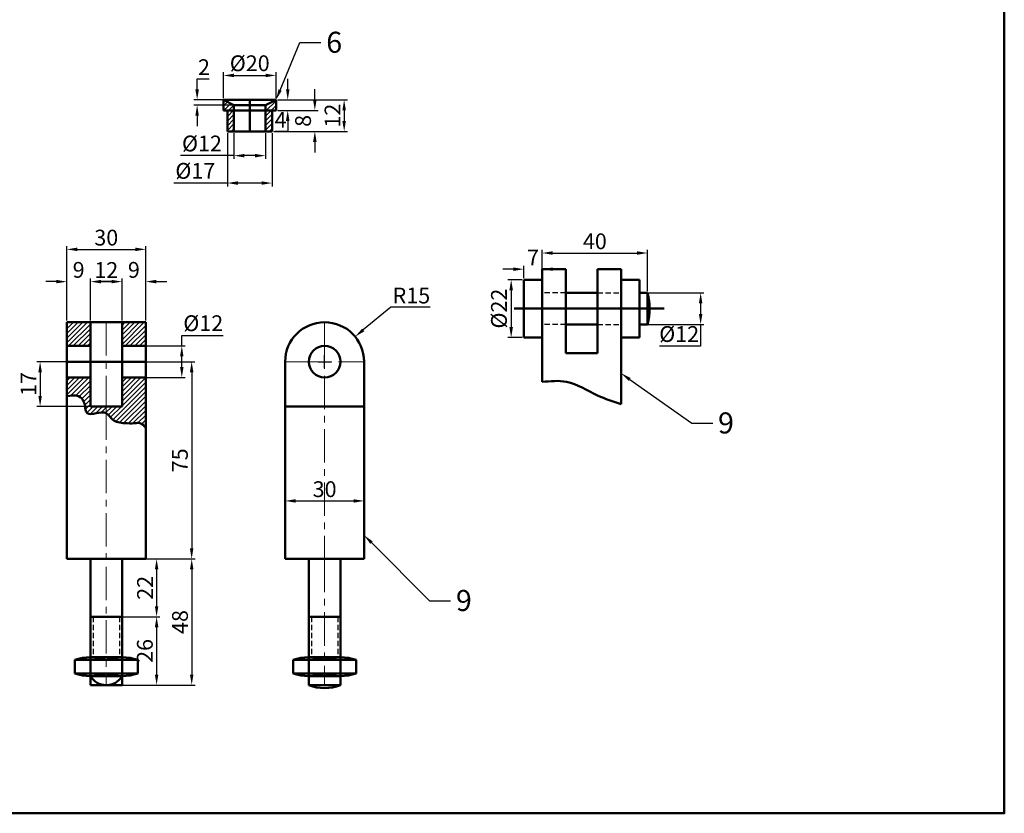
# Model space of a CAD drawing. Units: millimetres. Extents: x -266 to 493, y 251 to 855.
# Tile 2 of 3: x 118 to 493, y 251 to 553. Entities that reach past the tile are written whole.
import ezdxf
from ezdxf import colors
from ezdxf.entities.mleader import LeaderData, LeaderLine
from ezdxf.math import Vec2, Vec3

# ---------------------------------------------------------------- set-up
doc = ezdxf.new("R2010")
doc.units = ezdxf.units.MM
doc.header["$LTSCALE"] = 0.4
doc.linetypes.add('CENTER', pattern=[50.8, 31.75, -6.35, 6.35, -6.35])
doc.linetypes.add('DASHED', pattern=[19.05, 12.7, -6.35])
for name, color, linetype, lineweight in [('M-CNTR', 1, 'CENTER', 18), ('M-DIMS', 2, 'Continuous', 25), ('M-HATC', 8, 'Continuous', 18), ('M-HIDN', 3, 'DASHED', 25), ('M-OUTL', 7, 'Continuous', 50), ('M-TEXT', 7, 'Continuous', 25)]:
    doc.layers.add(name, color=color, linetype=linetype, lineweight=lineweight)
doc.styles.get("Standard").update_dxf_attribs({"font": 'arial.ttf'})
doc.dimstyles.new('ISO-25', dxfattribs={"dimtxt": 6, "dimasz": 4, "dimexe": 1.25, "dimexo": 0.625, "dimtad": 1, "dimtoh": 1, "dimtxsty": 'Standard', "dimcen": 2.5, "dimadec": 0, "dimazin": 0, "dimtfac": 1, "dimtofl": 0, "dimtmove": 0, "dimatfit": 3, "dimfxl": 1, "dimarcsym": 0})

# ---------------------------------------------------------------- blocks, each defined once
blk = doc.blocks.new('*D34')
at = {"layer": 'Defpoints', "color": 0, "transparency": 16777216}
for p in [(199.69, 510.13), (211.69, 510.13), (211.69, 500.9)]:
    blk.add_point(p, dxfattribs=at)
at = {"layer": 'M-DIMS', "color": 0, "lineweight": -2, "transparency": 16777216}
for p, q in [((199.69, 509.51), (199.69, 499.65)), ((211.69, 509.51), (211.69, 499.65)), ((199.69, 500.9), (179.38, 500.9)), ((207.69, 500.9), (203.69, 500.9))]:
    blk.add_line(p, q, dxfattribs=at)
at = {"layer": 'M-DIMS', "color": 0, "transparency": 16777216}
for points in [[(203.69, 501.57), (203.69, 500.23), (199.69, 500.9)], [(207.69, 501.57), (207.69, 500.23), (211.69, 500.9)]]:
    blk.add_solid(points, dxfattribs=at)
at = {"layer": 'M-DIMS', "color": 0, "transparency": 16777216, "insert": (187.53, 504.75), "char_height": 6, "attachment_point": 5}
blk.add_mtext('%%C12', dxfattribs=at)
blk = doc.blocks.new('*D35')
at = {"layer": 'Defpoints', "color": 0, "transparency": 16777216}
for p in [(197.19, 510.13), (214.19, 510.13), (214.19, 490.48)]:
    blk.add_point(p, dxfattribs=at)
at = {"layer": 'M-DIMS', "color": 0, "lineweight": -2, "transparency": 16777216}
for p, q in [((197.19, 509.51), (197.19, 489.23)), ((214.19, 509.51), (214.19, 489.23)), ((197.19, 490.48), (176.81, 490.48)), ((210.19, 490.48), (201.19, 490.48))]:
    blk.add_line(p, q, dxfattribs=at)
at = {"layer": 'M-DIMS', "color": 0, "transparency": 16777216}
for points in [[(201.19, 491.15), (201.19, 489.82), (197.19, 490.48)], [(210.19, 491.15), (210.19, 489.82), (214.19, 490.48)]]:
    blk.add_solid(points, dxfattribs=at)
at = {"layer": 'M-DIMS', "color": 0, "transparency": 16777216, "insert": (185, 494.34), "char_height": 6, "attachment_point": 5}
blk.add_mtext('%%C17', dxfattribs=at)
blk = doc.blocks.new('*D36')
at = {"layer": 'Defpoints', "color": 0, "transparency": 16777216}
for p in [(215.69, 522.13), (215.69, 518.13), (220.13, 518.13)]:
    blk.add_point(p, dxfattribs=at)
at = {"layer": 'M-DIMS', "color": 0, "lineweight": -2, "transparency": 16777216}
for p, q in [((220.13, 526.13), (220.13, 530.13)), ((216.31, 522.13), (221.38, 522.13)), ((216.31, 518.13), (221.38, 518.13)), ((220.13, 514.13), (220.13, 510.13)), ((220.13, 510.13), (215.36, 510.13))]:
    blk.add_line(p, q, dxfattribs=at)
at = {"layer": 'M-DIMS', "color": 0, "transparency": 16777216}
for points in [[(219.47, 526.13), (220.8, 526.13), (220.13, 522.13)], [(219.47, 514.13), (220.8, 514.13), (220.13, 518.13)]]:
    blk.add_solid(points, dxfattribs=at)
at = {"layer": 'M-DIMS', "color": 0, "transparency": 16777216, "insert": (217.43, 513.76), "char_height": 6, "attachment_point": 5}
blk.add_mtext('4', dxfattribs=at)
blk = doc.blocks.new('*D37')
at = {"layer": 'Defpoints', "color": 0, "transparency": 16777216}
for p in [(215.69, 522.13), (214.19, 510.13), (241.58, 510.13)]:
    blk.add_point(p, dxfattribs=at)
at = {"layer": 'M-DIMS', "color": 0, "lineweight": -2, "transparency": 16777216}
for p, q in [((216.31, 522.13), (242.83, 522.13)), ((241.58, 518.13), (241.58, 514.13)), ((214.81, 510.13), (242.83, 510.13))]:
    blk.add_line(p, q, dxfattribs=at)
at = {"layer": 'M-DIMS', "color": 0, "transparency": 16777216}
for points in [[(240.91, 518.13), (242.25, 518.13), (241.58, 522.13)], [(240.91, 514.13), (242.25, 514.13), (241.58, 510.13)]]:
    blk.add_solid(points, dxfattribs=at)
at = {"layer": 'M-DIMS', "color": 0, "transparency": 16777216, "insert": (237.94, 516.13), "char_height": 6, "attachment_point": 5, "rotation": 90}
blk.add_mtext('12', dxfattribs=at)
blk = doc.blocks.new('*D38')
at = {"layer": 'Defpoints', "color": 0, "transparency": 16777216}
for p in [(215.69, 518.13), (214.19, 510.13), (230.43, 510.13)]:
    blk.add_point(p, dxfattribs=at)
at = {"layer": 'M-DIMS', "color": 0, "lineweight": -2, "transparency": 16777216}
for p, q in [((230.43, 522.13), (230.43, 526.13)), ((216.31, 518.13), (231.68, 518.13)), ((214.81, 510.13), (231.68, 510.13)), ((230.43, 506.13), (230.43, 502.13))]:
    blk.add_line(p, q, dxfattribs=at)
at = {"layer": 'M-DIMS', "color": 0, "transparency": 16777216}
for points in [[(229.76, 522.13), (231.1, 522.13), (230.43, 518.13)], [(229.76, 506.13), (231.1, 506.13), (230.43, 510.13)]]:
    blk.add_solid(points, dxfattribs=at)
at = {"layer": 'M-DIMS', "color": 0, "transparency": 16777216, "insert": (226.74, 514.13), "char_height": 6, "attachment_point": 5, "rotation": 90}
blk.add_mtext('8', dxfattribs=at)
blk = doc.blocks.new('*D39')
at = {"layer": 'Defpoints', "color": 0, "transparency": 16777216}
for p in [(185.69, 522.14), (205.69, 522.14), (205.69, 520.14)]:
    blk.add_point(p, dxfattribs=at)
at = {"layer": 'M-DIMS', "color": 0, "lineweight": -2, "transparency": 16777216}
for p, q in [((185.69, 526.14), (185.69, 530.14)), ((185.69, 530.14), (190.29, 530.14)), ((205.06, 522.14), (184.44, 522.14)), ((205.06, 520.14), (184.44, 520.14)), ((185.69, 516.14), (185.69, 512.14))]:
    blk.add_line(p, q, dxfattribs=at)
at = {"layer": 'M-DIMS', "color": 0, "transparency": 16777216}
for points in [[(185.02, 526.14), (186.36, 526.14), (185.69, 522.14)], [(185.02, 516.14), (186.36, 516.14), (185.69, 520.14)]]:
    blk.add_solid(points, dxfattribs=at)
at = {"layer": 'M-DIMS', "color": 0, "transparency": 16777216, "insert": (188.3, 533.78), "char_height": 6, "attachment_point": 5}
blk.add_mtext('2', dxfattribs=at)
blk = doc.blocks.new('*D40')
at = {"layer": 'Defpoints', "color": 0, "transparency": 16777216}
for p in [(215.69, 531.4), (195.69, 522.13), (215.69, 522.13)]:
    blk.add_point(p, dxfattribs=at)
at = {"layer": 'M-DIMS', "color": 0, "lineweight": -2, "transparency": 16777216}
for p, q in [((195.69, 522.76), (195.69, 532.65)), ((215.69, 522.76), (215.69, 532.65)), ((199.69, 531.4), (211.69, 531.4))]:
    blk.add_line(p, q, dxfattribs=at)
at = {"layer": 'M-DIMS', "color": 0, "transparency": 16777216}
for points in [[(199.69, 532.07), (199.69, 530.74), (195.69, 531.4)], [(211.69, 532.07), (211.69, 530.74), (215.69, 531.4)]]:
    blk.add_solid(points, dxfattribs=at)
at = {"layer": 'M-DIMS', "color": 0, "transparency": 16777216, "insert": (205.69, 535.26), "char_height": 6, "attachment_point": 5}
blk.add_mtext('%%C20', dxfattribs=at)
blk = doc.blocks.new('*D41')
at = {"layer": 'Defpoints', "color": 0, "transparency": 16777216}
for p in [(162.53, 422.54), (162.53, 347.54), (183.62, 347.54)]:
    blk.add_point(p, dxfattribs=at)
at = {"layer": 'M-DIMS', "color": 0, "lineweight": -2, "transparency": 16777216}
for p, q in [((163.16, 422.54), (184.87, 422.54)), ((183.62, 418.54), (183.62, 351.54)), ((163.16, 347.54), (184.87, 347.54))]:
    blk.add_line(p, q, dxfattribs=at)
at = {"layer": 'M-DIMS', "color": 0, "transparency": 16777216}
for points in [[(182.95, 418.54), (184.28, 418.54), (183.62, 422.54)], [(182.95, 351.54), (184.28, 351.54), (183.62, 347.54)]]:
    blk.add_solid(points, dxfattribs=at)
at = {"layer": 'M-DIMS', "color": 0, "transparency": 16777216, "insert": (179.94, 385.04), "char_height": 6, "attachment_point": 5, "rotation": 90}
blk.add_mtext('75', dxfattribs=at)
blk = doc.blocks.new('*D42')
at = {"layer": 'Defpoints', "color": 0, "transparency": 16777216}
for p in [(151.16, 422.54), (126.01, 405.54), (151.16, 405.54)]:
    blk.add_point(p, dxfattribs=at)
at = {"layer": 'M-DIMS', "color": 0, "lineweight": -2, "transparency": 16777216}
for p, q in [((150.54, 422.54), (124.76, 422.54)), ((126.01, 418.54), (126.01, 409.54)), ((150.54, 405.54), (124.76, 405.54))]:
    blk.add_line(p, q, dxfattribs=at)
at = {"layer": 'M-DIMS', "color": 0, "transparency": 16777216}
for points in [[(125.35, 418.54), (126.68, 418.54), (126.01, 422.54)], [(125.35, 409.54), (126.68, 409.54), (126.01, 405.54)]]:
    blk.add_solid(points, dxfattribs=at)
at = {"layer": 'M-DIMS', "color": 0, "transparency": 16777216, "insert": (122.38, 414.04), "char_height": 6, "attachment_point": 5, "rotation": 90}
blk.add_mtext('17', dxfattribs=at)
blk = doc.blocks.new('*D43')
at = {"layer": 'Defpoints', "color": 0, "transparency": 16777216}
for p in [(161.66, 428.54), (179.87, 428.54), (161.66, 416.54)]:
    blk.add_point(p, dxfattribs=at)
at = {"layer": 'M-DIMS', "color": 0, "lineweight": -2, "transparency": 16777216}
for p, q in [((179.87, 428.54), (179.87, 432.54)), ((179.87, 432.54), (195.55, 432.54)), ((162.29, 428.54), (181.12, 428.54)), ((179.87, 420.54), (179.87, 424.54)), ((162.29, 416.54), (181.12, 416.54))]:
    blk.add_line(p, q, dxfattribs=at)
at = {"layer": 'M-DIMS', "color": 0, "transparency": 16777216}
for points in [[(179.2, 424.54), (180.53, 424.54), (179.87, 428.54)], [(179.2, 420.54), (180.53, 420.54), (179.87, 416.54)]]:
    blk.add_solid(points, dxfattribs=at)
at = {"layer": 'M-DIMS', "color": 0, "transparency": 16777216, "insert": (188.02, 436.4), "char_height": 6, "attachment_point": 5}
blk.add_mtext('%%C12', dxfattribs=at)
blk = doc.blocks.new('*D44')
at = {"layer": 'Defpoints', "color": 0, "transparency": 16777216}
for p in [(157.16, 347.54), (157.16, 325.54), (170.29, 325.54)]:
    blk.add_point(p, dxfattribs=at)
at = {"layer": 'M-DIMS', "color": 0, "lineweight": -2, "transparency": 16777216}
for p, q in [((157.79, 347.54), (171.54, 347.54)), ((170.29, 343.54), (170.29, 329.54)), ((157.79, 325.54), (171.54, 325.54))]:
    blk.add_line(p, q, dxfattribs=at)
at = {"layer": 'M-DIMS', "color": 0, "transparency": 16777216}
for points in [[(169.63, 343.54), (170.96, 343.54), (170.29, 347.54)], [(169.63, 329.54), (170.96, 329.54), (170.29, 325.54)]]:
    blk.add_solid(points, dxfattribs=at)
at = {"layer": 'M-DIMS', "color": 0, "transparency": 16777216, "insert": (166.66, 336.54), "char_height": 6, "attachment_point": 5, "rotation": 90}
blk.add_mtext('22', dxfattribs=at)
blk = doc.blocks.new('*D45')
at = {"layer": 'Defpoints', "color": 0, "transparency": 16777216}
for p in [(151.16, 325.54), (151.16, 299.54), (170.29, 299.54)]:
    blk.add_point(p, dxfattribs=at)
at = {"layer": 'M-DIMS', "color": 0, "lineweight": -2, "transparency": 16777216}
for p, q in [((151.79, 325.54), (171.54, 325.54)), ((170.29, 321.54), (170.29, 303.54)), ((151.79, 299.54), (171.54, 299.54))]:
    blk.add_line(p, q, dxfattribs=at)
at = {"layer": 'M-DIMS', "color": 0, "transparency": 16777216}
for points in [[(169.63, 321.54), (170.96, 321.54), (170.29, 325.54)], [(169.63, 303.54), (170.96, 303.54), (170.29, 299.54)]]:
    blk.add_solid(points, dxfattribs=at)
at = {"layer": 'M-DIMS', "color": 0, "transparency": 16777216, "insert": (166.6, 312.54), "char_height": 6, "attachment_point": 5, "rotation": 90}
blk.add_mtext('26', dxfattribs=at)
blk = doc.blocks.new('*D46')
at = {"layer": 'Defpoints', "color": 0, "transparency": 16777216}
for p in [(166.16, 347.54), (157.16, 299.54), (183.64, 299.54)]:
    blk.add_point(p, dxfattribs=at)
at = {"layer": 'M-DIMS', "color": 0, "lineweight": -2, "transparency": 16777216}
for p, q in [((166.79, 347.54), (184.89, 347.54)), ((183.64, 343.54), (183.64, 303.54)), ((157.79, 299.54), (184.89, 299.54))]:
    blk.add_line(p, q, dxfattribs=at)
at = {"layer": 'M-DIMS', "color": 0, "transparency": 16777216}
for points in [[(182.97, 343.54), (184.3, 343.54), (183.64, 347.54)], [(182.97, 303.54), (184.3, 303.54), (183.64, 299.54)]]:
    blk.add_solid(points, dxfattribs=at)
at = {"layer": 'M-DIMS', "color": 0, "transparency": 16777216, "insert": (179.95, 323.54), "char_height": 6, "attachment_point": 5, "rotation": 90}
blk.add_mtext('48', dxfattribs=at)
blk = doc.blocks.new('*D47')
at = {"layer": 'Defpoints', "color": 0, "transparency": 16777216}
for p in [(166.16, 465.26), (136.16, 437.54), (166.16, 437.54)]:
    blk.add_point(p, dxfattribs=at)
at = {"layer": 'M-DIMS', "color": 0, "lineweight": -2, "transparency": 16777216}
for p, q in [((136.16, 438.17), (136.16, 466.51)), ((140.16, 465.26), (162.16, 465.26)), ((166.16, 438.17), (166.16, 466.51))]:
    blk.add_line(p, q, dxfattribs=at)
at = {"layer": 'M-DIMS', "color": 0, "transparency": 16777216}
for points in [[(140.16, 465.93), (140.16, 464.6), (136.16, 465.26)], [(162.16, 465.93), (162.16, 464.6), (166.16, 465.26)]]:
    blk.add_solid(points, dxfattribs=at)
at = {"layer": 'M-DIMS', "color": 0, "transparency": 16777216, "insert": (151.16, 468.95), "char_height": 6, "attachment_point": 5}
blk.add_mtext('30', dxfattribs=at)
blk = doc.blocks.new('*D48')
at = {"layer": 'Defpoints', "color": 0, "transparency": 16777216}
for p in [(157.16, 452.99), (145.16, 437.54), (157.16, 437.54)]:
    blk.add_point(p, dxfattribs=at)
at = {"layer": 'M-DIMS', "color": 0, "lineweight": -2, "transparency": 16777216}
for p, q in [((145.16, 438.17), (145.16, 454.24)), ((149.16, 452.99), (153.16, 452.99)), ((157.16, 438.17), (157.16, 454.24))]:
    blk.add_line(p, q, dxfattribs=at)
at = {"layer": 'M-DIMS', "color": 0, "transparency": 16777216}
for points in [[(149.16, 453.66), (149.16, 452.33), (145.16, 452.99)], [(153.16, 453.66), (153.16, 452.33), (157.16, 452.99)]]:
    blk.add_solid(points, dxfattribs=at)
at = {"layer": 'M-DIMS', "color": 0, "transparency": 16777216, "insert": (151.16, 456.63), "char_height": 6, "attachment_point": 5}
blk.add_mtext('12', dxfattribs=at)
blk = doc.blocks.new('*D49')
at = {"layer": 'Defpoints', "color": 0, "transparency": 16777216}
for p in [(145.16, 452.99), (136.16, 437.54), (145.16, 437.54)]:
    blk.add_point(p, dxfattribs=at)
at = {"layer": 'M-DIMS', "color": 0, "lineweight": -2, "transparency": 16777216}
for p, q in [((132.16, 452.99), (128.16, 452.99)), ((136.16, 438.17), (136.16, 454.24)), ((145.16, 438.17), (145.16, 454.24)), ((149.16, 452.99), (153.16, 452.99))]:
    blk.add_line(p, q, dxfattribs=at)
at = {"layer": 'M-DIMS', "color": 0, "transparency": 16777216}
for points in [[(132.16, 453.66), (132.16, 452.33), (136.16, 452.99)], [(149.16, 453.66), (149.16, 452.33), (145.16, 452.99)]]:
    blk.add_solid(points, dxfattribs=at)
at = {"layer": 'M-DIMS', "color": 0, "transparency": 16777216, "insert": (140.66, 456.68), "char_height": 6, "attachment_point": 5}
blk.add_mtext('9', dxfattribs=at)
blk = doc.blocks.new('*D50')
at = {"layer": 'Defpoints', "color": 0, "transparency": 16777216}
for p in [(166.16, 452.99), (157.16, 437.54), (166.16, 437.54)]:
    blk.add_point(p, dxfattribs=at)
at = {"layer": 'M-DIMS', "color": 0, "lineweight": -2, "transparency": 16777216}
for p, q in [((153.16, 452.99), (149.16, 452.99)), ((157.16, 438.17), (157.16, 454.24)), ((166.16, 438.17), (166.16, 454.24)), ((170.16, 452.99), (174.16, 452.99))]:
    blk.add_line(p, q, dxfattribs=at)
at = {"layer": 'M-DIMS', "color": 0, "transparency": 16777216}
for points in [[(153.16, 453.66), (153.16, 452.33), (157.16, 452.99)], [(170.16, 453.66), (170.16, 452.33), (166.16, 452.99)]]:
    blk.add_solid(points, dxfattribs=at)
at = {"layer": 'M-DIMS', "color": 0, "transparency": 16777216, "insert": (161.66, 456.68), "char_height": 6, "attachment_point": 5}
blk.add_mtext('9', dxfattribs=at)
blk = doc.blocks.new('*D51')
at = {"layer": 'Defpoints', "color": 0, "transparency": 16777216}
for p in [(219.15, 379.25), (249.15, 379.25), (249.15, 369.59)]:
    blk.add_point(p, dxfattribs=at)
at = {"layer": 'M-DIMS', "color": 0, "lineweight": -2, "transparency": 16777216}
for p, q in [((219.15, 378.63), (219.15, 368.34)), ((249.15, 378.63), (249.15, 368.34)), ((223.15, 369.59), (245.15, 369.59))]:
    blk.add_line(p, q, dxfattribs=at)
at = {"layer": 'M-DIMS', "color": 0, "transparency": 16777216}
for points in [[(223.15, 370.25), (223.15, 368.92), (219.15, 369.59)], [(245.15, 370.25), (245.15, 368.92), (249.15, 369.59)]]:
    blk.add_solid(points, dxfattribs=at)
at = {"layer": 'M-DIMS', "color": 0, "transparency": 16777216, "insert": (234.15, 373.28), "char_height": 6, "attachment_point": 5}
blk.add_mtext('30', dxfattribs=at)
blk = doc.blocks.new('*D52')
at = {"layer": 'Defpoints', "color": 0, "transparency": 16777216}
for p in [(245.74, 432.07), (234.15, 422.54)]:
    blk.add_point(p, dxfattribs=at)
at = {"layer": 'M-DIMS', "color": 0, "lineweight": -2, "transparency": 16777216}
for p, q in [((259.32, 443.23), (248.83, 434.61)), ((274.33, 443.23), (259.32, 443.23)), ((234.15, 420.04), (234.15, 425.04)), ((231.65, 422.54), (236.65, 422.54))]:
    blk.add_line(p, q, dxfattribs=at)
at = {"layer": 'M-DIMS', "color": 0, "transparency": 16777216}
blk.add_solid([(248.41, 435.12), (249.25, 434.09), (245.74, 432.07)], dxfattribs=at)
at = {"layer": 'M-DIMS', "color": 0, "transparency": 16777216, "insert": (267.14, 446.92), "char_height": 6, "attachment_point": 5}
blk.add_mtext('R15', dxfattribs=at)
blk = doc.blocks.new('*D69')
at = {"layer": 'Defpoints', "color": 0, "ltscale": 0.4, "transparency": 16777216}
for p in [(356.87, 463.87), (316.87, 457.73), (356.87, 448.73)]:
    blk.add_point(p, dxfattribs=at)
at = {"layer": 'M-DIMS', "color": 0, "lineweight": -2, "ltscale": 0.4, "transparency": 16777216}
for p, q in [((316.87, 458.35), (316.87, 465.12)), ((356.87, 449.35), (356.87, 465.12)), ((320.87, 463.87), (352.87, 463.87))]:
    blk.add_line(p, q, dxfattribs=at)
at = {"layer": 'M-DIMS', "color": 0, "ltscale": 0.4, "transparency": 16777216}
for points in [[(320.87, 464.53), (320.87, 463.2), (316.87, 463.87)], [(352.87, 464.53), (352.87, 463.2), (356.87, 463.87)]]:
    blk.add_solid(points, dxfattribs=at)
at = {"layer": 'M-DIMS', "color": 0, "ltscale": 0.4, "transparency": 16777216, "insert": (336.87, 467.56), "char_height": 6, "attachment_point": 5}
blk.add_mtext('40', dxfattribs=at)
blk = doc.blocks.new('*D70')
at = {"layer": 'Defpoints', "color": 0, "ltscale": 0.4, "transparency": 16777216}
for p in [(316.87, 457.73), (309.87, 453.73), (316.87, 453.73)]:
    blk.add_point(p, dxfattribs=at)
at = {"layer": 'M-DIMS', "color": 0, "lineweight": -2, "ltscale": 0.4, "transparency": 16777216}
for p, q in [((305.87, 457.73), (301.87, 457.73)), ((309.87, 454.35), (309.87, 458.98)), ((316.87, 454.35), (316.87, 458.98)), ((320.87, 457.73), (324.87, 457.73))]:
    blk.add_line(p, q, dxfattribs=at)
at = {"layer": 'M-DIMS', "color": 0, "ltscale": 0.4, "transparency": 16777216}
for points in [[(305.87, 458.39), (305.87, 457.06), (309.87, 457.73)], [(320.87, 458.39), (320.87, 457.06), (316.87, 457.73)]]:
    blk.add_solid(points, dxfattribs=at)
at = {"layer": 'M-DIMS', "color": 0, "ltscale": 0.4, "transparency": 16777216, "insert": (313.37, 461.35), "char_height": 6, "attachment_point": 5}
blk.add_mtext('7', dxfattribs=at)
blk = doc.blocks.new('*D71')
at = {"layer": 'Defpoints', "color": 0, "ltscale": 0.4, "transparency": 16777216}
for p in [(309.87, 453.73), (305.06, 431.73), (309.87, 431.73)]:
    blk.add_point(p, dxfattribs=at)
at = {"layer": 'M-DIMS', "color": 0, "lineweight": -2, "ltscale": 0.4, "transparency": 16777216}
for p, q in [((309.24, 453.73), (303.81, 453.73)), ((305.06, 449.73), (305.06, 435.73)), ((309.24, 431.73), (303.81, 431.73))]:
    blk.add_line(p, q, dxfattribs=at)
at = {"layer": 'M-DIMS', "color": 0, "ltscale": 0.4, "transparency": 16777216}
for points in [[(304.39, 449.73), (305.73, 449.73), (305.06, 453.73)], [(304.39, 435.73), (305.73, 435.73), (305.06, 431.73)]]:
    blk.add_solid(points, dxfattribs=at)
at = {"layer": 'M-DIMS', "color": 0, "ltscale": 0.4, "transparency": 16777216, "insert": (301.2, 442.73), "char_height": 6, "attachment_point": 5, "rotation": 90}
blk.add_mtext('%%C22', dxfattribs=at)
blk = doc.blocks.new('*D72')
at = {"layer": 'Defpoints', "color": 0, "ltscale": 0.4, "transparency": 16777216}
for p in [(355.37, 448.73), (355.37, 436.73), (377.08, 436.73)]:
    blk.add_point(p, dxfattribs=at)
at = {"layer": 'M-DIMS', "color": 0, "lineweight": -2, "ltscale": 0.4, "transparency": 16777216}
for p, q in [((355.99, 448.73), (378.33, 448.73)), ((377.08, 444.73), (377.08, 440.73)), ((355.99, 436.73), (378.33, 436.73)), ((377.08, 436.73), (377.08, 428.43)), ((377.08, 428.43), (361.39, 428.43))]:
    blk.add_line(p, q, dxfattribs=at)
at = {"layer": 'M-DIMS', "color": 0, "ltscale": 0.4, "transparency": 16777216}
for points in [[(376.41, 444.73), (377.75, 444.73), (377.08, 448.73)], [(376.41, 440.73), (377.75, 440.73), (377.08, 436.73)]]:
    blk.add_solid(points, dxfattribs=at)
at = {"layer": 'M-DIMS', "color": 0, "ltscale": 0.4, "transparency": 16777216, "insert": (368.92, 432.28), "char_height": 6, "attachment_point": 5}
blk.add_mtext('%%C12', dxfattribs=at)
blk = doc.blocks.new('HEX-NUT')
at = {"ltscale": 0.4}
for p, q in [((0, 1), (0, 6.16)), ((0, 6.16), (24, 6.16)), ((24, 6.16), (24, 1)), ((24, 1), (0, 1))]:
    blk.add_line(p, q, dxfattribs=at)
for centre, start, end in [((6, -11.34), 71.0754, 108.9246), ((18, -11.34), 71.0754, 108.9246), ((6, 18.5), 251.0754, 288.9246), ((18, 18.5), 251.0754, 288.9246)]:
    blk.add_arc(centre, 18.5, start, end, dxfattribs=at)

msp = doc.modelspace()

# ---------------------------------------------------------------- hatches: boundary and pattern name
at = {"layer": 'M-HATC', "ltscale": 0.4}
h = msp.add_hatch(dxfattribs=at)
h.set_pattern_fill('ANSI31', color=256, scale=0.4)
h.set_pattern_definition([(45, (-1002.5745, 122.5025), (-0.8980256, 0.8980256), [])])
h.paths.add_polyline_path([(199.687, 518.134), (197.187, 518.134), (197.187, 510.134), (199.687, 510.134)])
h.paths.add_polyline_path([(199.687, 520.141), (195.687, 522.134), (195.687, 518.134), (199.687, 518.134)])
h.paths.add_polyline_path([(215.687, 522.134), (211.687, 520.141), (211.687, 518.134), (215.687, 518.134)])
h.paths.add_polyline_path([(214.187, 518.134), (211.687, 518.134), (211.687, 510.134), (214.187, 510.134)])
h = msp.add_hatch(dxfattribs=at)
h.set_pattern_fill('ANSI31', color=256, scale=0.4)
h.set_pattern_definition([(45, (-1040.6501, -343.0272), (-0.8980256, 0.8980256), [])])
edge = h.paths.add_edge_path()
edge.add_line((166.16, 416.544), (157.16, 416.544))
edge.add_line((157.16, 416.544), (157.16, 405.544))
edge.add_line((157.16, 405.544), (151.16, 405.544))
edge.add_line((151.16, 405.544), (151.16, 402.966))
edge.add_spline(control_points=[(151.16, 402.966), (152.119, 402.497), (153.527, 399.663), (157.911, 399.096), (161.304, 399.025), (164.34, 399.465), (165.488, 398.154), (166.16, 397.386)], knot_values=[19.1374251, 19.1374251, 19.1374251, 19.1374251, 22.4974265, 27.3616686, 31.1301945, 33.1279709, 35.9587534, 35.9587534, 35.9587534, 35.9587534], degree=3, periodic=0)
edge.add_line((166.16, 397.386), (166.16, 416.544))
edge = h.paths.add_edge_path()
edge.add_line((145.16, 416.544), (136.16, 416.544))
edge.add_line((136.16, 416.544), (136.16, 409.407))
edge.add_spline(control_points=[(136.16, 409.407), (137.727, 409.694), (140.265, 410.16), (143.38, 407.195), (142.762, 400.368), (149.096, 403.974), (151.16, 402.966)], knot_values=[0, 0, 0, 0, 4.4524591, 7.2118709, 11.9043741, 19.1374251, 19.1374251, 19.1374251, 19.1374251], degree=3, periodic=0)
edge.add_line((151.16, 402.966), (151.16, 405.544))
edge.add_line((151.16, 405.544), (145.16, 405.544))
edge.add_line((145.16, 405.544), (145.16, 416.544))
h.paths.add_polyline_path([(145.16, 437.544), (136.16, 437.544), (136.16, 428.544), (145.16, 428.544)])
h.paths.add_polyline_path([(166.16, 437.544), (157.16, 437.544), (157.16, 428.544), (166.16, 428.544)])

# ---------------------------------------------------------------- linework, layer by layer
at = {"layer": 'M-CNTR'}
msp.add_line((219.149, 422.544), (249.149, 422.544), dxfattribs=at)
for points in [[(151.16, 437.544), (151.16, 405.544), (151.16, 299.544)], [(234.149, 437.544), (234.149, 347.544), (234.149, 299.544)]]:
    msp.add_lwpolyline(points, dxfattribs=at)
at = {"layer": 'M-HIDN', "ltscale": 0.4}
for p, q in [((325.866, 448.728), (316.866, 448.728)), ((337.866, 448.728), (346.866, 448.728)), ((325.866, 436.728), (316.866, 436.728)), ((337.866, 436.728), (346.866, 436.728)), ((146.16, 325.544), (146.16, 310.139)), ((156.16, 325.544), (156.16, 310.139)), ((229.149, 325.544), (229.149, 310.139)), ((239.149, 325.544), (239.149, 310.139))]:
    msp.add_line(p, q, dxfattribs=at)
at = {"layer": 'M-OUTL'}
for p, q in [((195.687, 518.134), (195.687, 522.134)), ((215.687, 522.134), (195.687, 522.134)), ((199.687, 520.141), (195.687, 522.134)), ((205.687, 522.141), (205.687, 510.134)), ((211.687, 520.141), (215.687, 522.134)), ((215.687, 522.134), (215.687, 518.134)), ((215.687, 518.134), (195.687, 518.134)), ((197.187, 518.134), (197.187, 510.134)), ((199.687, 520.141), (211.687, 520.141)), ((199.687, 520.141), (199.687, 510.134)), ((211.687, 520.141), (211.687, 510.134)), ((214.187, 518.134), (214.187, 510.134)), ((197.187, 510.134), (214.187, 510.134)), ((325.866, 457.728), (316.866, 457.728)), ((325.866, 457.728), (325.866, 425.728)), ((337.866, 457.728), (337.866, 425.728)), ((346.866, 457.728), (337.866, 457.728)), ((363.267, 442.728), (306.221, 442.728)), ((136.16, 437.544), (136.16, 347.544)), ((166.16, 437.544), (136.16, 437.544)), ((145.16, 437.544), (145.16, 405.544)), ((157.16, 437.544), (157.16, 405.544)), ((166.16, 437.544), (166.16, 347.544)), ((337.866, 436.728), (325.866, 436.728)), ((145.16, 428.544), (136.16, 428.544)), ((166.16, 428.544), (157.16, 428.544)), ((337.866, 425.728), (325.866, 425.728)), ((166.16, 422.544), (136.16, 422.544)), ((219.149, 422.544), (219.149, 347.544)), ((249.149, 422.544), (249.149, 347.544)), ((145.16, 416.544), (136.16, 416.544)), ((166.16, 416.544), (157.16, 416.544)), ((157.16, 405.544), (145.16, 405.544)), ((219.149, 405.544), (249.149, 405.544)), ((226.649, 405.544), (241.649, 405.544)), ((226.649, 405.544), (241.649, 405.544)), ((166.16, 347.544), (136.16, 347.544)), ((145.16, 347.544), (145.16, 299.544)), ((157.16, 347.544), (157.16, 299.544)), ((219.149, 347.544), (249.149, 347.544)), ((228.149, 347.544), (228.149, 310.139)), ((240.149, 347.544), (240.149, 310.139)), ((157.16, 325.544), (145.16, 325.544)), ((228.149, 325.544), (240.149, 325.544)), ((157.16, 299.544), (145.16, 299.544)), ((228.149, 302.975), (228.149, 299.544)), ((228.149, 299.544), (240.149, 299.544)), ((240.149, 302.975), (240.149, 299.544))]:
    msp.add_line(p, q, dxfattribs=at)
at = {"layer": 'M-OUTL', "ltscale": 0.4}
for p, q in [((316.866, 457.728), (316.866, 414.865)), ((346.866, 457.728), (346.866, 406.43)), ((316.866, 453.728), (309.866, 453.728)), ((309.866, 453.728), (309.866, 431.728)), ((346.866, 453.728), (353.866, 453.728)), ((353.866, 453.728), (353.866, 431.728)), ((353.866, 448.728), (356.866, 448.728)), ((356.866, 448.728), (356.866, 442.728)), ((356.866, 442.728), (356.866, 436.728)), ((356.866, 436.728), (353.866, 436.728)), ((309.866, 431.728), (316.866, 431.728)), ((353.866, 431.728), (346.866, 431.728)), ((145.16, 325.544), (145.16, 310.139)), ((145.16, 310.139), (157.16, 310.139)), ((228.149, 310.139), (240.149, 310.139)), ((228.149, 310.139), (228.149, 302.975)), ((240.149, 310.139), (240.149, 302.975)), ((157.16, 302.975), (145.16, 302.975)), ((240.149, 302.975), (228.149, 302.975))]:
    msp.add_line(p, q, dxfattribs=at)
msp.add_lwpolyline([(-265.707, 854.992), (492.506, 854.992), (492.506, 250.777), (-265.707, 250.777)], close=True, dxfattribs=at)
at = {"layer": 'M-OUTL'}
msp.add_lwpolyline([(337.866, 448.728), (325.866, 448.728)], dxfattribs=at)
msp.add_circle((234.149, 422.544), 6, dxfattribs=at)
at = {"layer": 'M-OUTL', "ltscale": 0.4}
for centre, radius, start, end in [((335.134, 442.728), 22.545, 344.56575, 15.43425), ((151.16, 306.507), 6.963, 210.48753, 329.51247), ((234.149, 314.614), 16.22, 248.29009, 291.70991)]:
    msp.add_arc(centre, radius, start, end, dxfattribs=at)
at = {"layer": 'M-OUTL'}
msp.add_arc((234.149, 422.544), 15, 0, 180, dxfattribs=at)
at = {"layer": 'M-OUTL', "ltscale": 0.4}
for points, knots in [([(316.866, 414.865), (320, 415.156), (327.516, 415.854), (336.728, 409.66), (343.837, 407.395), (346.866, 406.43)], [0, 0, 0, 0, 9.2131006, 22.0944768, 31.656435, 31.656435, 31.656435, 31.656435]), ([(136.16, 409.407), (137.727, 409.694), (140.265, 410.16), (143.38, 407.195), (142.762, 400.368), (150.881, 404.99), (153.527, 399.663), (157.911, 399.096), (161.304, 399.025), (164.34, 399.465), (165.488, 398.154), (166.16, 397.386)], [0, 0, 0, 0, 4.4524591, 7.2118709, 11.9043741, 19.1374251, 22.4974265, 27.3616686, 31.1301945, 33.1279709, 35.9587534, 35.9587534, 35.9587534, 35.9587534])]:
    msp.add_open_spline(points, degree=3, knots=knots, dxfattribs=at)

# ---------------------------------------------------------------- block references
at = {"layer": 'M-OUTL', "rotation": 180}
msp.add_blockref('HEX-NUT', (163.16, 310.139), dxfattribs=at)
at = {"layer": 'M-OUTL'}
msp.add_blockref('HEX-NUT', (222.149, 302.975), dxfattribs=at)

# ---------------------------------------------------------------- dimensions: what is measured, and where the dimension line sits
at = {"layer": 'M-DIMS'}
dim = msp.add_linear_dim(base=(215.687, 531.403), p1=(195.687, 522.134), p2=(215.687, 522.134), text='%%C<>', dimstyle='ISO-25', override={"dimclrd": 0, "dimclre": 0, "dimclrt": 0}, dxfattribs=at)
dim.commit()
dim.dimension.update_dxf_attribs({"geometry": '*D40', "text_midpoint": (205.687, 535.259)})
for base, p1, p2, picture, middle in [((185.69, 522.141), (205.687, 520.141), (205.687, 522.141), '*D39', (188.302, 533.778)), ((220.133, 518.134), (215.687, 522.134), (215.687, 518.134), '*D36', (217.433, 513.759)), ((126.013, 405.544), (151.16, 422.544), (151.16, 405.544), '*D42', (122.376, 414.044)), ((183.617, 347.544), (162.534, 422.544), (162.534, 347.544), '*D41', (179.941, 385.044)), ((170.292, 325.544), (157.16, 347.544), (157.16, 325.544), '*D44', (166.655, 336.544)), ((183.637, 299.544), (166.16, 347.544), (157.16, 299.544), '*D46', (179.949, 323.544))]:
    dim = msp.add_linear_dim(base=base, p1=p1, p2=p2, angle=90, dimstyle='ISO-25', override={"dimclrd": 0, "dimclre": 0, "dimclrt": 0}, dxfattribs=at)
    dim.commit()
    dim.dimension.update_dxf_attribs({"geometry": picture, "text_midpoint": middle})
for base, p1, p2, picture, middle in [((230.429, 510.134), (215.687, 518.134), (214.187, 510.134), '*D38', (230.429, 514.134)), ((241.582, 510.134), (215.687, 522.134), (214.187, 510.134), '*D37', (241.582, 516.134)), ((170.292, 299.544), (151.16, 325.544), (151.16, 299.544), '*D45', (170.292, 312.544))]:
    dim = msp.add_linear_dim(base=base, p1=p1, p2=p2, angle=90, dimstyle='ISO-25', override={"dimclrd": 0, "dimclre": 0, "dimclrt": 0}, dxfattribs=at)
    dim.commit()
    dim.dimension.update_dxf_attribs({"geometry": picture, "text_midpoint": middle, "dimtype": 160})
for base, p1, p2, picture, middle in [((214.187, 490.483), (197.187, 510.134), (214.187, 510.134), '*D35', (185, 490.483)), ((211.687, 500.899), (199.687, 510.134), (211.687, 510.134), '*D34', (187.531, 500.899))]:
    dim = msp.add_linear_dim(base=base, p1=p1, p2=p2, text='%%C<>', dimstyle='ISO-25', override={"dimclrd": 0, "dimclre": 0, "dimclrt": 0}, dxfattribs=at)
    dim.commit()
    dim.dimension.update_dxf_attribs({"geometry": picture, "text_midpoint": middle, "dimtype": 160})
for base, p1, p2, picture, middle in [((166.16, 465.263), (136.16, 437.544), (166.16, 437.544), '*D47', (151.16, 468.953)), ((145.16, 452.992), (136.16, 437.544), (145.16, 437.544), '*D49', (140.66, 456.68)), ((157.16, 452.992), (145.16, 437.544), (157.16, 437.544), '*D48', (151.16, 456.629)), ((166.16, 452.992), (157.16, 437.544), (166.16, 437.544), '*D50', (161.66, 456.68)), ((249.149, 369.588), (219.149, 379.254), (249.149, 379.254), '*D51', (234.149, 373.279))]:
    dim = msp.add_linear_dim(base=base, p1=p1, p2=p2, dimstyle='ISO-25', override={"dimclrd": 0, "dimclre": 0, "dimclrt": 0}, dxfattribs=at)
    dim.commit()
    dim.dimension.update_dxf_attribs({"geometry": picture, "text_midpoint": middle})
at = {"layer": 'M-DIMS', "ltscale": 0.4}
for base, p1, p2, picture, middle in [((356.866, 463.868), (316.866, 457.728), (356.866, 448.728), '*D69', (336.866, 467.557)), ((316.866, 457.728), (309.866, 453.728), (316.866, 453.728), '*D70', (313.366, 461.353))]:
    dim = msp.add_linear_dim(base=base, p1=p1, p2=p2, dimstyle='ISO-25', override={"dimclrd": 0, "dimclre": 0, "dimclrt": 0}, dxfattribs=at)
    dim.commit()
    dim.dimension.update_dxf_attribs({"geometry": picture, "text_midpoint": middle})
dim = msp.add_linear_dim(base=(305.059, 431.728), p1=(309.866, 453.728), p2=(309.866, 431.728), angle=90, text='%%C<>', dimstyle='ISO-25', override={"dimclrd": 0, "dimclre": 0, "dimclrt": 0}, dxfattribs=at)
dim.commit()
dim.dimension.update_dxf_attribs({"geometry": '*D71', "text_midpoint": (301.202, 442.728)})
at = {"layer": 'M-DIMS'}
dim = msp.add_radius_dim(center=(234.149, 422.544), mpoint=(245.738, 432.068), dimstyle='ISO-25', override={"dimclrd": 0, "dimclre": 0, "dimclrt": 0}, dxfattribs=at)
dim.commit()
dim.dimension.update_dxf_attribs({"geometry": '*D52', "text_midpoint": (267.138, 443.231), "dimtype": 164})
at = {"layer": 'M-DIMS', "ltscale": 0.4}
dim = msp.add_linear_dim(base=(377.08, 436.728), p1=(355.366, 448.728), p2=(355.366, 436.728), angle=90, text='%%C<>', dimstyle='ISO-25', override={"dimclrd": 0, "dimclre": 0, "dimclrt": 0}, dxfattribs=at)
dim.commit()
dim.dimension.update_dxf_attribs({"geometry": '*D72', "text_midpoint": (368.925, 428.429), "dimtype": 160})
at = {"layer": 'M-DIMS'}
dim = msp.add_linear_dim(base=(179.867, 428.544), p1=(161.66, 416.544), p2=(161.66, 428.544), angle=90, text='%%C<>', dimstyle='ISO-25', override={"dimclrd": 0, "dimclre": 0, "dimclrt": 0}, dxfattribs=at)
dim.commit()
dim.dimension.update_dxf_attribs({"geometry": '*D43', "text_midpoint": (188.023, 436.401)})

# ---------------------------------------------------------------- leaders
at = {"layer": 'M-TEXT', "ltscale": 0.4}
ml = msp.add_multileader_mtext('Standard', dxfattribs=at)
ml.set_content('6', color=256)
ml.set_leader_properties()
ml.build(insert=Vec2(0, 0))
ctx = ml.context
ctx.base_point, ctx.char_height, ctx.plane_origin = Vec3(232.761, 543.954), 8, Vec3(215.687, 522.134)
notes = []
notes.append((ctx, [(0, (1, 1, 0), (224.761, 543.954), (1, 0), 8, [(0, [(215.687, 522.134)], 0, [])])]))
ctx.mtext.insert, ctx.mtext.flow_direction = Vec3(234.761, 548.022), 5
ml = msp.add_multileader_mtext('Standard', dxfattribs=at)
ml.set_content('9', color=256)
ml.set_leader_properties()
ml.build(insert=Vec2(0, 0))
ctx = ml.context
ctx.base_point, ctx.char_height, ctx.plane_origin = Vec3(381.674, 399.177), 8, Vec3(346.866, 418.113)
notes.append((ctx, [(0, (1, 1, 0), (373.674, 399.177), (1, 0), 8, [(0, [(346.866, 418.113)], 0, [])])]))
ctx.mtext.insert, ctx.mtext.flow_direction = Vec3(383.674, 403.245), 5
ml = msp.add_multileader_mtext('Standard', dxfattribs=at)
ml.set_content('9', color=256)
ml.set_leader_properties()
ml.build(insert=Vec2(0, 0))
ctx = ml.context
ctx.base_point, ctx.char_height, ctx.plane_origin = Vec3(282.057, 331.651), 8, Vec3(249.149, 356.558)
notes.append((ctx, [(0, (1, 1, 0), (274.057, 331.651), (1, 0), 8, [(0, [(249.149, 356.558)], 0, [])])]))
ctx.mtext.insert, ctx.mtext.flow_direction = Vec3(284.057, 335.719), 5
for ctx, leaders in notes:
    for number, flags, end, landing, length, lines in leaders:
        leader = LeaderData()
        leader.index, (leader.has_last_leader_line, leader.has_dogleg_vector, leader.attachment_direction) = number, flags
        leader.last_leader_point, leader.dogleg_vector, leader.dogleg_length = Vec3(end), Vec3(landing), length
        for number, points, colour, breaks in lines:
            line = LeaderLine()
            line.index, line.vertices, line.color, line.breaks = number, Vec3.list(points), colors.encode_raw_color(colour), breaks
            leader.lines.append(line)
        ctx.leaders.append(leader)

doc.saveas('drawing.dxf')
